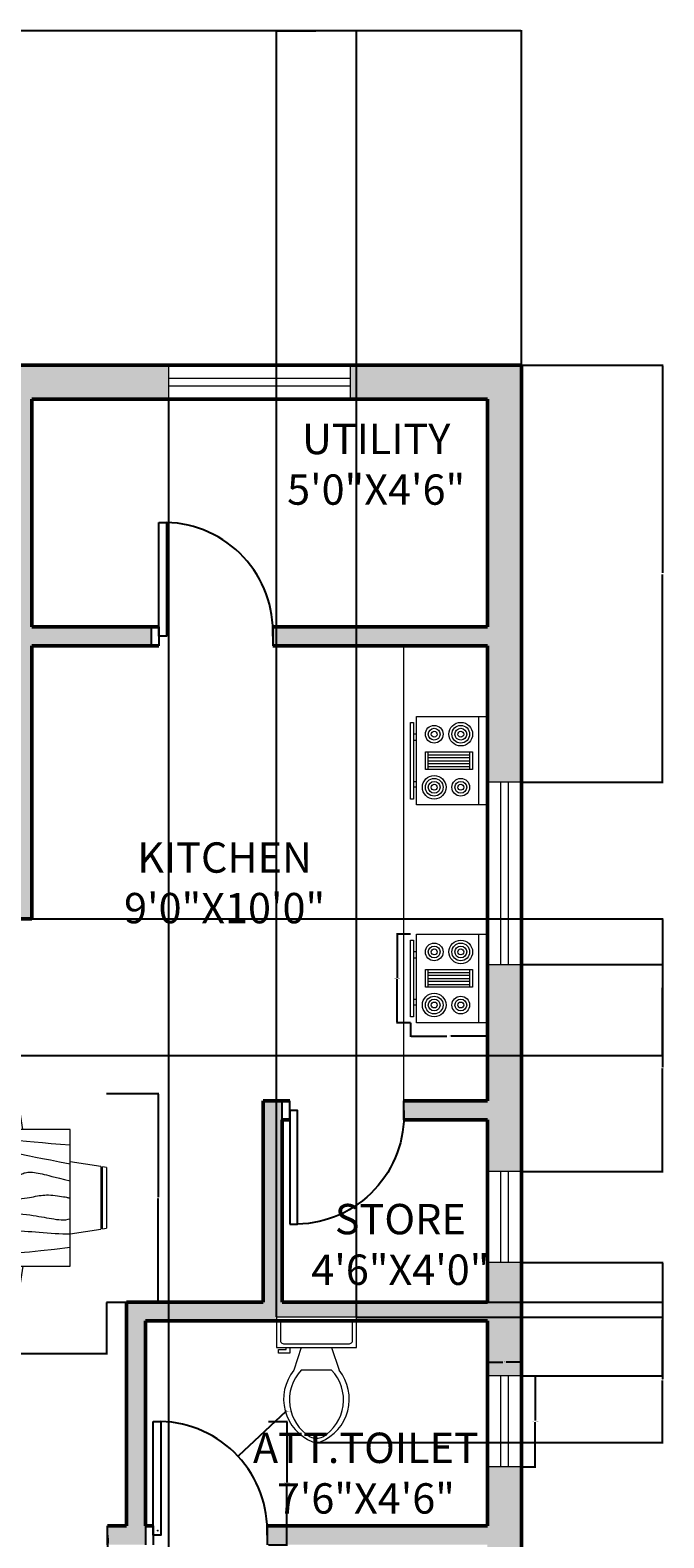
# Model space of a CAD drawing. Units: inches. Extents: x 76 to 532, y 199 to 998.
# Tile 4 of 4: x 365 to 532, y 601 to 998. Entities that reach past the tile are written whole.
import ezdxf

# ---------------------------------------------------------------- set-up
doc = ezdxf.new("R2010")
doc.units = ezdxf.units.IN
for name, color, linetype, lineweight in [('A-ANNO-DIMS', 2, 'Continuous', 18), ('A-AREA-IDEN', 3, 'Continuous', 18), ('A-EQPM', 8, 'Continuous', 18), ('A-FLOR-FIXT', 8, 'Continuous', 18), ('A-FURN', 8, 'Continuous', 18), ('A-WALL', 7, 'Continuous', 50), ('A-WALL-PATT', 45, 'Continuous', 13), ('doors', 1, 'Continuous', 25), ('windows', 140, 'Continuous', 18)]:
    doc.layers.add(name, color=color, linetype=linetype, lineweight=lineweight)
doc.styles.get("Standard").update_dxf_attribs({"font": 'arial.ttf'})
doc.dimstyles.get("Standard").update_dxf_attribs({"dimtxt": 0.18, "dimasz": 0.18, "dimexe": 0.18, "dimexo": 0.0625, "dimgap": 0.09, "dimtad": 0, "dimtih": 1, "dimtoh": 1, "dimdec": 4, "dimzin": 0, "dimdsep": 46, "dimtxsty": 'Standard', "dimcen": 0.09, "dimadec": 0, "dimazin": 0, "dimtfac": 1, "dimtdec": 4, "dimtofl": 0, "dimtmove": 0, "dimatfit": 3, "dimfxl": 1, "dimtolj": 1, "dimtzin": 0, "dimarcsym": 0})

# ---------------------------------------------------------------- blocks, each defined once
blk = doc.blocks.new('Dining Set - 36 x 72 in.')
for p, q in [((-22.2343, 26.00059), (-23.4847, 17.99762)), ((-22.2304, 26), (-5.7608, 26)), ((-22, 27.5), (-22.1562, 26.50042)), ((-5.8416, 26.5), (-22.1534, 26.5)), ((-22, 27.5), (-6, 27.5)), ((-5.8437, 26.49966), (-6, 27.5)), ((-4.5152, 17.99762), (-5.7655, 25.99926)), ((5.7657, 26.00059), (4.5153, 17.99762)), ((5.7696, 26), (22.2392, 26)), ((6, 27.5), (5.8438, 26.50042)), ((22.1584, 26.5), (5.8466, 26.5)), ((6, 27.5), (22, 27.5)), ((22.1563, 26.49966), (22, 27.5)), ((23.4848, 17.99762), (22.2345, 25.99926)), ((36, 18), (-36, 18)), ((-36, 18), (-36, -18)), ((36, -18), (36, 18)), ((-45.5, 8), (-44.5004, 8.15617)), ((-45.5, 8), (-45.5, -8)), ((-44.5, -8.15843), (-44.5, 8.15338)), ((-44.0006, 8.23428), (-35.9976, 9.48474)), ((-44, 8.23041), (-44, -8.23915)), ((44.0006, 8.23428), (35.9976, 9.48474)), ((44, 8.23041), (44, -8.23915)), ((44.5, -8.15843), (44.5, 8.15338)), ((45.5, 8), (44.5005, 8.15617)), ((45.5, 8), (45.5, -8)), ((-44.4997, -8.15631), (-45.5, -8)), ((-35.9976, -9.48476), (-43.9993, -8.2345)), ((35.9976, -9.48476), (43.9993, -8.2345)), ((44.4997, -8.15631), (45.5, -8)), ((-36, -18), (36, -18)), ((-22.2343, -26.0006), (-23.4847, -17.99762)), ((-4.5152, -17.99762), (-5.7655, -25.99928)), ((5.7657, -26.0006), (4.5153, -17.99762)), ((23.4848, -17.99762), (22.2345, -25.99928)), ((-22.2304, -26), (-5.7608, -26)), ((-22, -27.5), (-22.1562, -26.50044)), ((-5.8416, -26.5), (-22.1534, -26.5)), ((-22, -27.5), (-6, -27.5)), ((-5.8437, -26.49967), (-6, -27.5)), ((5.7696, -26), (22.2392, -26)), ((6, -27.5), (5.8438, -26.50044)), ((22.1584, -26.5), (5.8466, -26.5)), ((6, -27.5), (22, -27.5)), ((22.1563, -26.49967), (22, -27.5))]:
    blk.add_line(p, q)
for points in [[(-36, 15), (-31.1772, 14.97754), (-26.8079, 14.91406), (-22.8538, 14.81543), (-19.276, 14.6875), (-16.0362, 14.53613), (-13.0957, 14.36718), (-10.4159, 14.18652), (-7.9583, 14), (-5.6904, 13.81315), (-3.6035, 13.63021), (-1.6954, 13.45508), (0.0365, 13.29166), (1.5945, 13.14388), (2.9811, 13.01562), (4.1988, 12.9108), (5.25, 12.83333), (6.1393, 12.78613), (6.8802, 12.76823), (7.4883, 12.77767), (7.9792, 12.8125), (8.3685, 12.87077), (8.6719, 12.95052), (8.9049, 13.0498), (9.0833, 13.16666), (9.2205, 13.29899), (9.3216, 13.44401), (9.3895, 13.59879), (9.4271, 13.76041), (9.4373, 13.92594), (9.4232, 14.09245), (9.3875, 14.257), (9.3333, 14.41666), (9.2638, 14.56917), (9.1836, 14.71484), (9.0975, 14.85465), (9.0104, 14.98958), (8.9272, 15.1206), (8.8529, 15.2487), (8.7922, 15.37483), (8.75, 15.5), (8.7305, 15.62467), (8.7344, 15.74739), (8.7617, 15.86621), (8.8125, 15.97916), (8.8867, 16.08431), (8.9844, 16.17968), (9.1055, 16.26334), (9.25, 16.33333), (9.4189, 16.38802), (9.6172, 16.42708), (9.8506, 16.45052), (10.125, 16.45833), (10.4463, 16.45052), (10.8203, 16.42708), (11.2529, 16.38802), (11.75, 16.33333), (12.3184, 16.26318), (12.9694, 16.17838), (13.7151, 16.07991), (14.5677, 15.96875), (15.5395, 15.84586), (16.6426, 15.71224), (17.8893, 15.56884), (19.2917, 15.41666), (20.859, 15.25667), (22.5879, 15.08984), (24.4721, 14.91715), (26.5052, 14.73958), (28.6809, 14.5581), (30.9929, 14.3737), (33.4347, 14.18733), (36, 14)], [(-36, 10), (-28.9766, 10.14274), (-23.1725, 10.20442), (-18.4241, 10.19775), (-14.5677, 10.13541), (-11.4399, 10.03011), (-8.877, 9.89453), (-6.7154, 9.74137), (-4.7917, 9.58333), (-2.9698, 9.43082), (-1.2246, 9.28515), (0.4415, 9.14534), (2.026, 9.01041), (3.5266, 8.87939), (4.9408, 8.7513), (6.266, 8.62516), (7.5, 8.5), (8.6411, 8.37549), (9.6914, 8.2539), (10.6538, 8.13818), (11.5312, 8.03125), (12.3267, 7.93603), (13.043, 7.85547), (13.6831, 7.79248), (14.25, 7.75), (14.7471, 7.7303), (15.1797, 7.73307), (15.5537, 7.75732), (15.875, 7.80208), (16.1494, 7.86637), (16.3828, 7.94922), (16.5811, 8.04964), (16.75, 8.16666), (16.8944, 8.29915), (17.0143, 8.44531), (17.1089, 8.60319), (17.1771, 8.77083), (17.218, 8.94629), (17.2305, 9.1276), (17.2137, 9.31282), (17.1667, 9.5), (17.0895, 9.6875), (16.987, 9.875), (16.8649, 10.0625), (16.7292, 10.25), (16.5856, 10.4375), (16.4401, 10.625), (16.2985, 10.8125), (16.1667, 11), (16.05, 11.18733), (15.9518, 11.3737), (15.8752, 11.5581), (15.8229, 11.73958), (15.798, 11.91715), (15.8034, 12.08984), (15.842, 12.25667), (15.9167, 12.41666), (16.0295, 12.56836), (16.1784, 12.70833), (16.3605, 12.83268), (16.5729, 12.9375), (16.8127, 13.01888), (17.0768, 13.07291), (17.3625, 13.0957), (17.6667, 13.08333), (17.9894, 13.03312), (18.3418, 12.94726), (18.7382, 12.82918), (19.1927, 12.68229), (19.7195, 12.51001), (20.3327, 12.31575), (21.0465, 12.10294), (21.875, 11.875), (22.8357, 11.63354), (23.959, 11.37304), (25.2786, 11.08618), (26.8282, 10.76562), (28.6414, 10.40405), (30.752, 9.99414), (33.1936, 9.52856), (36, 9)], [(-36, 5.5), (-30.7157, 5.3348), (-26.069, 5.20963), (-21.9946, 5.11767), (-18.4271, 5.05208), (-15.3009, 5.00602), (-12.5508, 4.97265), (-10.1112, 4.94515), (-7.9167, 4.91666), (-5.909, 4.88167), (-4.0586, 4.83984), (-2.3429, 4.79215), (-0.7396, 4.73958), (0.7739, 4.6831), (2.22, 4.6237), (3.6213, 4.56233), (5, 4.5), (6.373, 4.43782), (7.7344, 4.3776), (9.0723, 4.32129), (10.375, 4.27083), (11.6309, 4.22819), (12.8281, 4.19531), (13.9551, 4.17415), (15, 4.16666), (15.954, 4.17448), (16.819, 4.19791), (17.6001, 4.23698), (18.3021, 4.29166), (18.9299, 4.36198), (19.4883, 4.44791), (19.9823, 4.54948), (20.4167, 4.66666), (20.7969, 4.79899), (21.1302, 4.94401), (21.4245, 5.09879), (21.6875, 5.26041), (21.9271, 5.42594), (22.1511, 5.59245), (22.3672, 5.757), (22.5834, 5.91666), (22.8065, 6.06868), (23.0404, 6.21093), (23.2879, 6.34147), (23.5521, 6.45833), (23.8358, 6.55957), (24.142, 6.64323), (24.4735, 6.70735), (24.8334, 6.75), (25.2235, 6.76969), (25.642, 6.76692), (26.0858, 6.74267), (26.5521, 6.69791), (27.0379, 6.63362), (27.5404, 6.55078), (28.0565, 6.45036), (28.5834, 6.33333), (29.1242, 6.19987), (29.7071, 6.04687), (30.3661, 5.87044), (31.1354, 5.66666), (32.0493, 5.43164), (33.142, 5.16146), (34.4475, 4.85221), (36, 4.5)], [(-36, -1), (-30.7915, -0.6591), (-26.0195, -0.38216), (-21.6519, -0.16284), (-17.6563, 0.00521), (-14.0005, 0.12833), (-10.6523, 0.21289), (-7.5796, 0.26522), (-4.75, 0.29166), (-2.134, 0.29793), (0.2878, 0.28711), (2.5317, 0.26163), (4.6146, 0.22396), (6.5529, 0.17651), (8.3633, 0.12174), (10.0623, 0.06209), (11.6667, 0), (13.1899, -0.06201), (14.6341, -0.1211), (15.9982, -0.17432), (17.2813, -0.21875), (18.4823, -0.25147), (19.6003, -0.26953), (20.6343, -0.27002), (21.5834, -0.25), (22.4481, -0.20768), (23.2357, -0.14584), (23.9549, -0.06836), (24.6146, 0.02083), (25.2235, 0.11784), (25.7904, 0.21875), (26.3241, 0.31966), (26.8334, 0.41666), (27.3265, 0.50618), (27.8099, 0.58593), (28.2894, 0.65397), (28.7709, 0.70833), (29.2601, 0.74707), (29.763, 0.76823), (30.2855, 0.76985), (30.8334, 0.75), (31.4088, 0.70784), (31.9994, 0.64713), (32.589, 0.57275), (33.1615, 0.48958), (33.7008, 0.4025), (34.1908, 0.3164), (34.6153, 0.23616), (34.9584, 0.16666), (35.2099, 0.11165), (35.3848, 0.07031), (35.504, 0.04069), (35.5886, 0.02083), (35.6594, 0.00879), (35.7377, 0.0026), (35.8442, 0.00032), (36, 0)], [(-36, -6.5), (-27.1843, -6.31267), (-20.084, -6.1263), (-14.469, -5.9419), (-10.1094, -5.76042), (-6.7752, -5.58285), (-4.2363, -5.41016), (-2.2629, -5.24333), (-0.625, -5.08334), (0.8708, -4.93099), (2.2715, -4.78646), (3.5872, -4.64974), (4.8281, -4.52084), (6.0046, -4.39974), (7.127, -4.28646), (8.2053, -4.18099), (9.25, -4.08334), (10.2705, -3.99382), (11.2734, -3.91407), (12.2647, -3.84603), (13.25, -3.79167), (14.2354, -3.75293), (15.2266, -3.73177), (16.2295, -3.73015), (17.25, -3.75), (18.2912, -3.79248), (19.3451, -3.85547), (20.4009, -3.93604), (21.4479, -4.03125), (22.4754, -4.13819), (23.4727, -4.25391), (24.4289, -4.37549), (25.3334, -4.5), (26.1785, -4.62492), (26.9694, -4.74935), (27.7145, -4.87281), (28.4219, -4.99479), (29.1, -5.11483), (29.7572, -5.23242), (30.4016, -5.34709), (31.0417, -5.45834), (31.6837, -5.56437), (32.3262, -5.65821), (32.9658, -5.73153), (33.599, -5.77604), (34.2224, -5.78345), (34.8327, -5.74545), (35.4264, -5.65373), (36, -5.5)], [(-36, -10), (-26.4022, -9.81299), (-18.4675, -9.62891), (-11.9839, -9.45069), (-6.7396, -9.28125), (-2.5226, -9.12354), (0.8789, -8.98047), (3.6769, -8.85498), (6.0833, -8.75), (8.2767, -8.66765), (10.3021, -8.60677), (12.1712, -8.56543), (13.8958, -8.54167), (15.4876, -8.53353), (16.9583, -8.53907), (18.3197, -8.55632), (19.5834, -8.58334), (20.7616, -8.61841), (21.8685, -8.66081), (22.9188, -8.71004), (23.9271, -8.76563), (24.9081, -8.82707), (25.8763, -8.89388), (26.8465, -8.96558), (27.8334, -9.04167), (28.8474, -9.12118), (29.8828, -9.20117), (30.93, -9.27824), (31.9792, -9.34896), (33.0205, -9.40991), (34.0443, -9.45768), (35.0407, -9.48885), (36, -9.5)], [(-36, -14.5), (-30.0881, -14.33513), (-25.0332, -14.21224), (-20.7312, -14.12647), (-17.0781, -14.07292), (-13.97, -14.04671), (-11.3027, -14.04297), (-8.9724, -14.05681), (-6.875, -14.08334), (-4.9224, -14.11833), (-3.0905, -14.16016), (-1.3709, -14.20785), (0.2448, -14.26042), (1.7647, -14.3169), (3.1973, -14.3763), (4.5507, -14.43767), (5.8333, -14.5), (7.0554, -14.5621), (8.235, -14.62175), (9.3922, -14.67652), (10.5469, -14.72396), (11.7192, -14.76164), (12.929, -14.78711), (14.1965, -14.79794), (15.5417, -14.79167), (16.9933, -14.76424), (18.6152, -14.70508), (20.4804, -14.60197), (22.6615, -14.44271), (25.2312, -14.21509), (28.2624, -13.9069), (31.8277, -13.50594), (36, -13)]]:
    blk.add_lwpolyline(points)
blk = doc.blocks.new('Range-Oven - 30 in top')
for p, q in [((0, -3), (30, -3)), ((12, -6), (18, -6)), ((13, -20), (13, -6)), ((14, -6), (14, -20)), ((15, -20), (15, -6)), ((16, -6), (16, -20)), ((17, -20), (17, -6)), ((18, -20), (12, -20)), ((6, -24), (6, -25)), ((8, -25), (8, -24)), ((22, -25), (22, -24)), ((24, -24), (24, -25))]:
    blk.add_line(p, q)
for points in [[(0, -24), (0, 0), (30, 0), (30, -24)], [(12, -21), (12, -5), (18, -5), (18, -21)], [(2, -26), (2, -25), (28, -25), (28, -26)]]:
    blk.add_lwpolyline(points, close=True)
for centre, radius in [((6, -9), 4), ((6, -9), 3), ((6, -9), 2), ((6, -9), 1), ((24, -9), 3), ((24, -9), 2), ((24, -9), 1), ((6, -18), 3), ((24, -18), 4), ((24, -18), 3), ((6, -18), 2), ((6, -18), 1), ((24, -18), 2), ((24, -18), 1)]:
    blk.add_circle(centre, radius)
blk = doc.blocks.new('*U10')
for p, q in [((9.5, -6), (9.5, -2)), ((-10, -8.5), (-8, -8.5)), ((-10, -9.5), (-10, -8.5)), ((-7, -9.5), (-10, -9.5)), ((-8, -8.5), (-8, -8)), ((-7, -8), (-7, -9.5)), ((-4, -8), (-6, -14)), ((4, -8), (6, -14)), ((4, -14), (-4, -14))]:
    blk.add_line(p, q)
blk.add_lwpolyline([(10.5, -8), (10.5, 0), (-10.5, 0), (-10.5, -8)], close=True)
for points in [[(-9.5, -2), (-9.5, -6)], [(8.5, -1), (-8.5, -1)], [(-8.5, -7), (8.5, -7)]]:
    blk.add_lwpolyline(points)
for centre, radius, start, end in [((-8.62, -1.88), 0.884, 81.8699, 188.1301), ((8.62, -1.88), 0.884, 351.8699, 98.1301), ((-8.62, -6.12), 0.884, 171.8699, 278.1301), ((8.62, -6.12), 0.884, 261.8699, 8.1301), ((3.52, -21.58), 12.17, 141.4691, 247.9714), ((4.2, -21.82), 11.33, 136.3677, 238.9468), ((-3.52, -21.58), 12.17, 292.0284, 38.5307), ((-4.2, -21.82), 11.33, 301.053, 43.6321), ((0, -27.88), 4, 245.7318, 294.2682), ((0, -29), 4, 254.8605, 285.1395)]:
    blk.add_arc(centre, radius, start, end)
blk = doc.blocks.new('glass')
at = {"layer": 'windows'}
for p, q in [((-12, 5.5), (-12, -3.5)), ((12, 5.5), (12, -3.5)), ((-12, 2), (12, 2)), ((-12, 0), (12, 0))]:
    blk.add_line(p, q, dxfattribs=at)
blk = doc.blocks.new('DOOR-SWING-30IN')
for p, q in [((0, 5), (0, 0)), ((2, 5), (2, 0)), ((32, 5), (32, 0))]:
    blk.add_line(p, q)
blk.add_lwpolyline([(2, 32.5), (4, 32.5), (4, 2.5), (2, 2.5)], close=True)
blk.add_arc((3.27, 3.75), 28.76, 357.5089, 88.5412)
blk = doc.blocks.new('WIN-48IN')
for p, q in [((0, 5.5), (48, 5.5)), ((0, 3.5), (48, 3.5))]:
    blk.add_line(p, q)
blk.add_lwpolyline([(0, 0), (48, 0), (48, 9), (0, 9)], close=True)
blk = doc.blocks.new('*D15')
at = {"layer": 'A-ANNO-DIMS', "color": 0, "lineweight": -2, "transparency": 16777216}
for p, q in [((428.25, 631.53), (433.25, 631.53)), ((433.07, 631.35), (433.07, 615.46)), ((433.07, 599.21), (433.07, 615.09)), ((428.25, 599.03), (433.25, 599.03))]:
    blk.add_line(p, q, dxfattribs=at)
at = {"layer": 'A-ANNO-DIMS', "color": 0, "transparency": 16777216}
for points in [[(433.04, 631.35), (433.1, 631.35), (433.07, 631.53)], [(433.04, 599.21), (433.1, 599.21), (433.07, 599.03)]]:
    blk.add_solid(points, dxfattribs=at)
at = {"layer": 'Defpoints', "color": 0, "transparency": 16777216}
for p in [(428.19, 631.53), (433.07, 631.53), (428.19, 599.03)]:
    blk.add_point(p, dxfattribs=at)
at = {"layer": 'A-ANNO-DIMS', "color": 0, "transparency": 16777216, "insert": (433.07, 615.28), "char_height": 0.18, "attachment_point": 5}
blk.add_mtext('\\A1;DOOR 33 TYP.', dxfattribs=at)
blk = doc.blocks.new('*D19')
at = {"layer": 'A-ANNO-DIMS', "color": 0, "lineweight": -2, "transparency": 16777216}
for p, q in [((494.92, 643.58), (498.64, 643.58)), ((498.46, 643.4), (498.46, 631.76)), ((498.46, 619.76), (498.46, 631.39)), ((494.92, 619.58), (498.64, 619.58))]:
    blk.add_line(p, q, dxfattribs=at)
at = {"layer": 'A-ANNO-DIMS', "color": 0, "transparency": 16777216}
for points in [[(498.43, 643.4), (498.49, 643.4), (498.46, 643.58)], [(498.43, 619.76), (498.49, 619.76), (498.46, 619.58)]]:
    blk.add_solid(points, dxfattribs=at)
at = {"layer": 'Defpoints', "color": 0, "transparency": 16777216}
for p in [(494.86, 643.58), (494.86, 619.58), (498.46, 619.58)]:
    blk.add_point(p, dxfattribs=at)
at = {"layer": 'A-ANNO-DIMS', "color": 0, "transparency": 16777216, "insert": (498.46, 631.58), "char_height": 0.18, "attachment_point": 5}
blk.add_mtext('\\A1;GLAZING 24 TYP.', dxfattribs=at)
blk = doc.blocks.new('*D20')
at = {"layer": 'A-ANNO-DIMS', "color": 0, "lineweight": -2, "transparency": 16777216}
for p, q in [((485.86, 643.64), (485.86, 647.36)), ((486.04, 647.18), (489.9, 647.18)), ((494.68, 647.18), (490.82, 647.18)), ((494.86, 643.64), (494.86, 647.36))]:
    blk.add_line(p, q, dxfattribs=at)
at = {"layer": 'A-ANNO-DIMS', "color": 0, "transparency": 16777216}
for points in [[(486.04, 647.21), (486.04, 647.15), (485.86, 647.18)], [(494.68, 647.21), (494.68, 647.15), (494.86, 647.18)]]:
    blk.add_solid(points, dxfattribs=at)
at = {"layer": 'Defpoints', "color": 0, "transparency": 16777216}
for p in [(494.86, 647.18), (485.86, 643.58), (494.86, 643.58)]:
    blk.add_point(p, dxfattribs=at)
at = {"layer": 'A-ANNO-DIMS', "color": 0, "transparency": 16777216, "insert": (490.36, 647.18), "char_height": 0.18, "attachment_point": 5}
blk.add_mtext('\\A1;9 TYP.', dxfattribs=at)
blk = doc.blocks.new('*D23')
at = {"layer": 'A-ANNO-DIMS', "color": 0, "lineweight": -2, "transparency": 16777216}
for p, q in [((465.58, 759.98), (461.96, 759.98)), ((462.14, 759.8), (462.14, 748.5)), ((462.14, 736.83), (462.14, 748.13)), ((465.58, 736.65), (461.96, 736.65))]:
    blk.add_line(p, q, dxfattribs=at)
at = {"layer": 'A-ANNO-DIMS', "color": 0, "transparency": 16777216}
for points in [[(462.11, 759.8), (462.17, 759.8), (462.14, 759.98)], [(462.11, 736.83), (462.17, 736.83), (462.14, 736.65)]]:
    blk.add_solid(points, dxfattribs=at)
at = {"layer": 'Defpoints', "color": 0, "transparency": 16777216}
for p in [(465.64, 759.98), (462.14, 736.65), (465.64, 736.65)]:
    blk.add_point(p, dxfattribs=at)
at = {"layer": 'A-ANNO-DIMS', "color": 0, "transparency": 16777216, "insert": (462.14, 748.31), "char_height": 0.18, "attachment_point": 5}
blk.add_mtext('\\A1;RANGE 23 TYP.', dxfattribs=at)
blk = doc.blocks.new('*D24')
at = {"layer": 'A-ANNO-DIMS', "color": 0, "lineweight": -2, "transparency": 16777216}
for p, q in [((465.64, 736.59), (465.64, 732.97)), ((485.86, 736.59), (485.86, 732.97)), ((465.82, 733.15), (475.22, 733.15)), ((485.68, 733.15), (476.28, 733.15))]:
    blk.add_line(p, q, dxfattribs=at)
at = {"layer": 'A-ANNO-DIMS', "color": 0, "transparency": 16777216}
for points in [[(465.82, 733.18), (465.82, 733.12), (465.64, 733.15)], [(485.68, 733.18), (485.68, 733.12), (485.86, 733.15)]]:
    blk.add_solid(points, dxfattribs=at)
at = {"layer": 'Defpoints', "color": 0, "transparency": 16777216}
for p in [(465.64, 736.65), (485.86, 736.65), (485.86, 733.15)]:
    blk.add_point(p, dxfattribs=at)
at = {"layer": 'A-ANNO-DIMS', "color": 0, "transparency": 16777216, "insert": (475.75, 733.15), "char_height": 0.18, "attachment_point": 5}
blk.add_mtext('\\A1;20 TYP.', dxfattribs=at)
blk = doc.blocks.new('*D29')
at = {"layer": 'A-ANNO-DIMS', "color": 0, "lineweight": -2, "transparency": 16777216}
for p, q in [((294.53, 662.92), (294.53, 649.15)), ((385.53, 662.92), (385.53, 649.15)), ((294.71, 649.33), (339.08, 649.33)), ((385.35, 649.33), (340.98, 649.33))]:
    blk.add_line(p, q, dxfattribs=at)
at = {"layer": 'A-ANNO-DIMS', "color": 0, "transparency": 16777216}
for points in [[(294.71, 649.36), (294.71, 649.3), (294.53, 649.33)], [(385.35, 649.36), (385.35, 649.3), (385.53, 649.33)]]:
    blk.add_solid(points, dxfattribs=at)
at = {"layer": 'Defpoints', "color": 0, "transparency": 16777216}
for p in [(294.53, 662.98), (385.53, 662.98), (385.53, 649.33)]:
    blk.add_point(p, dxfattribs=at)
at = {"layer": 'A-ANNO-DIMS', "color": 0, "transparency": 16777216, "insert": (340.03, 649.33), "char_height": 0.18, "attachment_point": 5}
blk.add_mtext('\\A1;DINING SET 91', dxfattribs=at)
blk = doc.blocks.new('*D30')
at = {"layer": 'A-ANNO-DIMS', "color": 0, "lineweight": -2, "transparency": 16777216}
for p, q in [((385.59, 717.98), (399.36, 717.98)), ((399.18, 717.8), (399.18, 690.66)), ((399.18, 663.16), (399.18, 690.3)), ((385.59, 662.98), (399.36, 662.98))]:
    blk.add_line(p, q, dxfattribs=at)
at = {"layer": 'A-ANNO-DIMS', "color": 0, "transparency": 16777216}
for points in [[(399.15, 717.8), (399.21, 717.8), (399.18, 717.98)], [(399.15, 663.16), (399.21, 663.16), (399.18, 662.98)]]:
    blk.add_solid(points, dxfattribs=at)
at = {"layer": 'Defpoints', "color": 0, "transparency": 16777216}
for p in [(385.53, 717.98), (399.18, 717.98), (385.53, 662.98)]:
    blk.add_point(p, dxfattribs=at)
at = {"layer": 'A-ANNO-DIMS', "color": 0, "transparency": 16777216, "insert": (399.18, 690.48), "char_height": 0.18, "attachment_point": 5}
blk.add_mtext('\\A1;55', dxfattribs=at)
blk = doc.blocks.new('*D31')
at = {"layer": 'A-ANNO-DIMS', "color": 0, "lineweight": -2, "transparency": 16777216}
for p, q in [((160.86, 910.09), (160.86, 998.31)), ((161.04, 998.13), (327.57, 998.13)), ((494.68, 998.13), (328.15, 998.13)), ((494.86, 910.09), (494.86, 998.31))]:
    blk.add_line(p, q, dxfattribs=at)
at = {"layer": 'A-ANNO-DIMS', "color": 0, "transparency": 16777216}
for points in [[(161.04, 998.16), (161.04, 998.1), (160.86, 998.13)], [(494.68, 998.16), (494.68, 998.1), (494.86, 998.13)]]:
    blk.add_solid(points, dxfattribs=at)
at = {"layer": 'Defpoints', "color": 0, "transparency": 16777216}
for p in [(494.86, 998.13), (160.86, 910.03), (494.86, 910.03)]:
    blk.add_point(p, dxfattribs=at)
at = {"layer": 'A-ANNO-DIMS', "color": 0, "transparency": 16777216, "insert": (327.86, 998.13), "char_height": 0.18, "attachment_point": 5}
blk.add_mtext('\\A1;334', dxfattribs=at)
blk = doc.blocks.new('*D34')
at = {"layer": 'A-ANNO-DIMS', "color": 0, "lineweight": -2, "transparency": 16777216}
for p, q in [((494.92, 910.03), (532.14, 910.03)), ((531.96, 909.85), (531.96, 855.21)), ((531.96, 800.21), (531.96, 854.85)), ((494.92, 800.03), (532.14, 800.03))]:
    blk.add_line(p, q, dxfattribs=at)
at = {"layer": 'A-ANNO-DIMS', "color": 0, "transparency": 16777216}
for points in [[(531.93, 909.85), (531.99, 909.85), (531.96, 910.03)], [(531.93, 800.21), (531.99, 800.21), (531.96, 800.03)]]:
    blk.add_solid(points, dxfattribs=at)
at = {"layer": 'Defpoints', "color": 0, "transparency": 16777216}
for p in [(494.86, 910.03), (531.96, 910.03), (494.86, 800.03)]:
    blk.add_point(p, dxfattribs=at)
at = {"layer": 'A-ANNO-DIMS', "color": 0, "transparency": 16777216, "insert": (531.96, 855.03), "char_height": 0.18, "attachment_point": 5}
blk.add_mtext('\\A1;110', dxfattribs=at)
blk = doc.blocks.new('*D35')
at = {"layer": 'A-ANNO-DIMS', "color": 0, "lineweight": -2, "transparency": 16777216}
for p, q in [((494.92, 752.03), (532.14, 752.03)), ((531.96, 751.85), (531.96, 724.93)), ((531.96, 697.65), (531.96, 724.57)), ((494.92, 697.47), (532.14, 697.47))]:
    blk.add_line(p, q, dxfattribs=at)
at = {"layer": 'A-ANNO-DIMS', "color": 0, "transparency": 16777216}
for points in [[(531.93, 751.85), (531.99, 751.85), (531.96, 752.03)], [(531.93, 697.65), (531.99, 697.65), (531.96, 697.47)]]:
    blk.add_solid(points, dxfattribs=at)
at = {"layer": 'Defpoints', "color": 0, "transparency": 16777216}
for p in [(494.86, 752.03), (531.96, 752.03), (494.86, 697.47)]:
    blk.add_point(p, dxfattribs=at)
at = {"layer": 'A-ANNO-DIMS', "color": 0, "transparency": 16777216, "insert": (531.96, 724.75), "char_height": 0.18, "attachment_point": 5}
blk.add_mtext('\\A1;54.55', dxfattribs=at)
blk = doc.blocks.new('*D36')
at = {"layer": 'A-ANNO-DIMS', "color": 0, "lineweight": -2, "transparency": 16777216}
for p, q in [((494.92, 673.47), (532.14, 673.47)), ((531.96, 673.29), (531.96, 658.71)), ((531.96, 643.76), (531.96, 658.34)), ((494.92, 643.58), (532.14, 643.58))]:
    blk.add_line(p, q, dxfattribs=at)
at = {"layer": 'A-ANNO-DIMS', "color": 0, "transparency": 16777216}
for points in [[(531.93, 673.29), (531.99, 673.29), (531.96, 673.47)], [(531.93, 643.76), (531.99, 643.76), (531.96, 643.58)]]:
    blk.add_solid(points, dxfattribs=at)
at = {"layer": 'Defpoints', "color": 0, "transparency": 16777216}
for p in [(494.86, 673.47), (494.86, 643.58), (531.96, 643.58)]:
    blk.add_point(p, dxfattribs=at)
at = {"layer": 'A-ANNO-DIMS', "color": 0, "transparency": 16777216, "insert": (531.96, 658.53), "char_height": 0.18, "attachment_point": 5}
blk.add_mtext('\\A1;29.895', dxfattribs=at)
blk = doc.blocks.new('*D41')
at = {"layer": 'A-ANNO-DIMS', "color": 0, "lineweight": -2, "transparency": 16777216}
for p, q in [((347.36, 900.97), (347.36, 198.6)), ((401.86, 900.97), (401.86, 198.6)), ((347.54, 198.78), (374.28, 198.78)), ((401.68, 198.78), (374.93, 198.78))]:
    blk.add_line(p, q, dxfattribs=at)
at = {"layer": 'A-ANNO-DIMS', "color": 0, "transparency": 16777216}
for points in [[(347.54, 198.81), (347.54, 198.75), (347.36, 198.78)], [(401.68, 198.81), (401.68, 198.75), (401.86, 198.78)]]:
    blk.add_solid(points, dxfattribs=at)
at = {"layer": 'Defpoints', "color": 0, "transparency": 16777216}
for p in [(347.36, 901.03), (401.86, 901.03), (401.86, 198.78)]:
    blk.add_point(p, dxfattribs=at)
at = {"layer": 'A-ANNO-DIMS', "color": 0, "transparency": 16777216, "insert": (374.61, 198.78), "char_height": 0.18, "attachment_point": 5}
blk.add_mtext('\\A1;54.5', dxfattribs=at)
blk = doc.blocks.new('*D46')
at = {"layer": 'A-ANNO-DIMS', "color": 0, "lineweight": -2, "transparency": 16777216}
for p, q in [((249.92, 764.03), (532.14, 764.03)), ((531.96, 763.85), (531.96, 746.21)), ((531.96, 728.21), (531.96, 745.85)), ((249.92, 728.03), (532.14, 728.03))]:
    blk.add_line(p, q, dxfattribs=at)
at = {"layer": 'A-ANNO-DIMS', "color": 0, "transparency": 16777216}
for points in [[(531.93, 763.85), (531.99, 763.85), (531.96, 764.03)], [(531.93, 728.21), (531.99, 728.21), (531.96, 728.03)]]:
    blk.add_solid(points, dxfattribs=at)
at = {"layer": 'Defpoints', "color": 0, "transparency": 16777216}
for p in [(249.86, 764.03), (531.96, 764.03), (249.86, 728.03)]:
    blk.add_point(p, dxfattribs=at)
at = {"layer": 'A-ANNO-DIMS', "color": 0, "transparency": 16777216, "insert": (531.96, 746.03), "char_height": 0.18, "attachment_point": 5}
blk.add_mtext('\\A1;36', dxfattribs=at)
blk = doc.blocks.new('*D48')
at = {"layer": 'A-ANNO-DIMS', "color": 0, "lineweight": -2, "transparency": 16777216}
for p, q in [((430.36, 659.09), (430.36, 998.31)), ((430.54, 998.13), (440.65, 998.13)), ((451.18, 998.13), (441.06, 998.13)), ((451.36, 659.09), (451.36, 998.31))]:
    blk.add_line(p, q, dxfattribs=at)
at = {"layer": 'A-ANNO-DIMS', "color": 0, "transparency": 16777216}
for points in [[(430.54, 998.16), (430.54, 998.1), (430.36, 998.13)], [(451.18, 998.16), (451.18, 998.1), (451.36, 998.13)]]:
    blk.add_solid(points, dxfattribs=at)
at = {"layer": 'Defpoints', "color": 0, "transparency": 16777216}
for p in [(451.36, 998.13), (430.36, 659.03), (451.36, 659.03)]:
    blk.add_point(p, dxfattribs=at)
at = {"layer": 'A-ANNO-DIMS', "color": 0, "transparency": 16777216, "insert": (440.86, 998.13), "char_height": 0.18, "attachment_point": 5}
blk.add_mtext('\\A1;21', dxfattribs=at)
blk = doc.blocks.new('*D49')
at = {"layer": 'A-ANNO-DIMS', "color": 0, "lineweight": -2, "transparency": 16777216}
for p, q in [((485.92, 663.03), (532.14, 663.03)), ((531.96, 662.85), (531.96, 653.48)), ((531.96, 643.76), (531.96, 653.12)), ((494.92, 643.58), (532.14, 643.58))]:
    blk.add_line(p, q, dxfattribs=at)
at = {"layer": 'A-ANNO-DIMS', "color": 0, "transparency": 16777216}
for points in [[(531.93, 662.85), (531.99, 662.85), (531.96, 663.03)], [(531.93, 643.76), (531.99, 643.76), (531.96, 643.58)]]:
    blk.add_solid(points, dxfattribs=at)
at = {"layer": 'Defpoints', "color": 0, "transparency": 16777216}
for p in [(485.86, 663.03), (531.96, 663.03), (494.86, 643.58)]:
    blk.add_point(p, dxfattribs=at)
at = {"layer": 'A-ANNO-DIMS', "color": 0, "transparency": 16777216, "insert": (531.96, 653.3), "char_height": 0.18, "attachment_point": 5}
blk.add_mtext('\\A1;19.45', dxfattribs=at)
blk = doc.blocks.new('*D55')
at = {"layer": 'A-ANNO-DIMS', "color": 0, "lineweight": -2, "transparency": 16777216}
for p, q in [((451.42, 659.03), (532.14, 659.03)), ((531.96, 658.85), (531.96, 642.71)), ((531.96, 626.21), (531.96, 642.35)), ((440.92, 626.03), (532.14, 626.03))]:
    blk.add_line(p, q, dxfattribs=at)
at = {"layer": 'A-ANNO-DIMS', "color": 0, "transparency": 16777216}
for points in [[(531.93, 658.85), (531.99, 658.85), (531.96, 659.03)], [(531.93, 626.21), (531.99, 626.21), (531.96, 626.03)]]:
    blk.add_solid(points, dxfattribs=at)
at = {"layer": 'Defpoints', "color": 0, "transparency": 16777216}
for p in [(451.36, 659.03), (440.86, 626.03), (531.96, 626.03)]:
    blk.add_point(p, dxfattribs=at)
at = {"layer": 'A-ANNO-DIMS', "color": 0, "transparency": 16777216, "insert": (531.96, 642.53), "char_height": 0.18, "attachment_point": 5}
blk.add_mtext('\\A1;33', dxfattribs=at)
blk = doc.blocks.new('*D60')
at = {"layer": 'A-ANNO-DIMS', "color": 0, "lineweight": -2, "transparency": 16777216}
for p, q in [((432.76, 634.17), (420.28, 622.52)), ((432.94, 634.17), (432.76, 634.17)), ((399.03, 602.78), (399.21, 602.78)), ((399.12, 602.69), (399.12, 602.87))]:
    blk.add_line(p, q, dxfattribs=at)
at = {"layer": 'A-ANNO-DIMS', "color": 0, "transparency": 16777216}
blk.add_solid([(420.26, 622.55), (420.3, 622.5), (420.15, 622.4)], dxfattribs=at)
at = {"layer": 'Defpoints', "color": 0, "transparency": 16777216}
for p in [(420.15, 622.4), (399.12, 602.78)]:
    blk.add_point(p, dxfattribs=at)
at = {"layer": 'A-ANNO-DIMS', "color": 0, "transparency": 16777216, "insert": (433.62, 634.17), "char_height": 0.18, "attachment_point": 5}
blk.add_mtext('\\A1;3X R28.76', dxfattribs=at)

msp = doc.modelspace()

# ---------------------------------------------------------------- hatches: boundary and pattern name
at = {"layer": 'A-WALL-PATT'}
h = msp.add_hatch(color=256, dxfattribs=at)
h.dxf.hatch_style = 1
h.paths.add_polyline_path([(323.3571, 910.0275), (259.8571, 910.0275), (259.8571, 901.0275), (301.8571, 901.0275), (301.8571, 769.0275), (301.8571, 764.0275), (306.8571, 764.0275), (306.8571, 806.0275), (306.8571, 811.0275), (306.8571, 901.0275), (323.3571, 901.0275)])
h.paths.add_polyline_path([(211.8571, 910.0275), (160.8571, 910.0275), (160.8571, 539.5719), (169.8571, 539.5719), (169.8571, 599.0275), (263.8571, 599.0275), (263.8571, 604.0275), (169.8571, 604.0275), (169.8571, 764.0275), (263.8571, 764.0275), (263.8571, 766.5275, -0.0179874), (263.8571, 769.0275), (169.8571, 769.0275), (169.8571, 901.0275), (211.8571, 901.0275)])
h.paths.add_polyline_path([(401.8571, 910.0275), (347.3571, 910.0275), (347.3571, 901.0275), (360.8571, 901.0275), (360.8571, 811.0275), (338.8571, 811.0275, -0.02174236), (338.8571, 808.5275), (338.8571, 806.0275), (360.8571, 806.0275), (360.8571, 764.0275), (365.8571, 764.0275), (365.8571, 836.0275), (397.3621, 836.0275), (397.3621, 841.0275), (365.8571, 841.0275), (365.8571, 901.0275), (401.8571, 901.0275)])
h.paths.add_polyline_path([(169.8571, 479.5719), (160.8571, 479.5719), (160.8571, 434.0275), (211.8571, 434.0275), (211.8571, 443.0275), (169.8571, 443.0275)])
h.paths.add_polyline_path([(310.8571, 443.0275), (259.8571, 443.0275), (259.8571, 434.0275), (310.8571, 434.0275), (310.8571, 438.5275, -0.03336892)])
h.paths.add_polyline_path([(353.8571, 599.0275), (353.8571, 604.0275), (348.8571, 604.0275), (348.8571, 599.0275), (348.8571, 443.0275), (348.8571, 434.0275), (396.8571, 434.0275), (396.8571, 443.0275), (353.8571, 443.0275)])
h.paths.add_polyline_path([(494.8571, 619.5776), (485.8571, 619.5776), (485.8571, 604.0275), (427.8571, 604.0275, -0.02174236), (427.8571, 601.5275), (427.8571, 599.0275), (485.8571, 599.0275), (485.8571, 443.0275), (444.8571, 443.0275), (444.8571, 434.0275), (494.8571, 434.0275)])
h.paths.add_polyline_path([(494.8571, 673.4729), (485.8571, 673.4729), (485.8571, 663.0275), (431.8571, 663.0275), (431.8571, 711.0275), (431.8571, 716.0275), (426.8571, 716.0275), (426.8571, 663.0275), (390.8571, 663.0275), (390.8571, 604.0275), (385.8571, 604.0275), (385.8571, 601.5275, -0.02174236), (385.8571, 599.0275), (395.8571, 599.0275), (395.8571, 604.0275), (395.8571, 658.0275), (430.3571, 658.0275), (430.3571, 659.0275), (451.3571, 659.0275), (451.3571, 658.0275), (485.8571, 658.0275), (485.8571, 643.5776), (494.8571, 643.5776)])
h.paths.add_polyline_path([(494.8571, 752.0275), (485.8571, 752.0275), (485.8571, 716.0275), (463.8571, 716.0275), (463.8571, 713.5275, -0.02174236), (463.8571, 711.0275), (485.8571, 711.0275), (485.8571, 697.4729), (494.8571, 697.4729)])
h.paths.add_polyline_path([(494.8571, 910.0275), (449.8571, 910.0275), (449.8571, 901.0275), (485.8571, 901.0275), (485.8571, 841.0275), (429.3621, 841.0275, -0.02174236), (429.3621, 838.5275), (429.3621, 836.0275), (485.8571, 836.0275), (485.8571, 800.0275), (494.8571, 800.0275)])

# ---------------------------------------------------------------- linework, layer by layer
at = {"layer": 'A-FLOR-FIXT'}
msp.add_line((463.8571, 716.0275), (463.8571, 836.0275), dxfattribs=at)
at = {"layer": 'A-WALL'}
for p, q in [((494.8571, 910.0275), (160.8571, 910.0275)), ((494.8571, 910.0275), (494.8571, 434.0275)), ((485.8571, 901.0275), (365.8571, 901.0275)), ((365.8571, 901.0275), (365.8571, 841.0275)), ((485.8571, 901.0275), (485.8571, 841.0275)), ((399.3621, 841.0275), (365.8571, 841.0275)), ((485.8571, 841.0275), (429.3621, 841.0275)), ((365.8571, 836.0275), (365.8571, 764.0275)), ((399.3621, 836.0275), (365.8571, 836.0275)), ((485.8571, 836.0275), (429.3621, 836.0275)), ((485.8571, 836.0275), (485.8571, 716.0275)), ((365.8571, 764.0275), (360.8571, 764.0275)), ((426.8571, 716.0275), (426.8571, 663.0275)), ((433.8571, 716.0275), (426.8571, 716.0275)), ((485.8571, 716.0275), (463.8571, 716.0275)), ((431.8571, 711.0275), (431.8571, 663.0275)), ((433.8571, 711.0275), (431.8571, 711.0275)), ((485.8571, 711.0275), (463.8571, 711.0275)), ((485.8571, 711.0275), (485.8571, 663.0275)), ((390.8571, 663.0275), (390.8571, 604.0275)), ((426.8571, 663.0275), (390.8571, 663.0275)), ((485.8571, 663.0275), (431.8571, 663.0275)), ((485.8571, 658.0275), (395.8571, 658.0275)), ((395.8571, 658.0275), (395.8571, 604.0275)), ((485.8571, 658.0275), (485.8571, 604.0275)), ((390.8571, 604.0275), (385.8571, 604.0275)), ((397.8571, 604.0275), (395.8571, 604.0275)), ((485.8571, 604.0275), (427.8571, 604.0275))]:
    msp.add_line(p, q, dxfattribs=at)

# ---------------------------------------------------------------- block references
at = {"layer": 'A-EQPM', "xscale": 0.777460115447206, "yscale": 0.777460115447206, "zscale": 0.777460115447206, "rotation": 270}
for p in [(485.8571, 817.3774), (485.8571, 759.9753)]:
    msp.add_blockref('Range-Oven - 30 in top', p, dxfattribs=at)
at = {"layer": 'A-FLOR-FIXT'}
msp.add_blockref('*U10', (440.8571, 659.0275), dxfattribs=at)
at = {"layer": 'A-FURN'}
msp.add_blockref('Dining Set - 36 x 72 in.', (340.0288, 690.4778), dxfattribs=at)
at = {"layer": 'doors'}
for p in [(397.3621, 836.0275), (395.8571, 599.0275)]:
    msp.add_blockref('DOOR-SWING-30IN', p, dxfattribs=at)
at = {"layer": 'doors', "extrusion": (0, 0, -1), "zscale": -1, "rotation": 180}
for p in [(-431.8571, 716.0275), (-353.8571, 604.0275)]:
    msp.add_blockref('DOOR-SWING-30IN', p, dxfattribs=at)
at = {"layer": 'windows'}
msp.add_blockref('WIN-48IN', (401.8571, 901.0275), dxfattribs=at)
for name, p, rotation in [('WIN-48IN', (485.8571, 800.0275), 270.0000000000001), ('glass', (489.3571, 685.4729), 270), ('glass', (489.3571, 631.5776), 270)]:
    msp.add_blockref(name, p, dxfattribs=dict(at, rotation=rotation))

# ---------------------------------------------------------------- texts
at = {"layer": 'A-AREA-IDEN', "char_height": 8, "attachment_point": 1}
for s, insert in [('\\pxqc;UTILITY\\P5\'0"X4\'6"', (416.2705, 894.5345)), ('\\pxqc;KITCHEN\\P9\'0"X10\'0"', (376.3639, 784.1978)), ('\\pxqc;STORE\\P4\'6"X4\'0"', (422.6414, 688.8795)), ('\\pxqc;ATT.TOILET\\P7\'6"X4\'6"', (413.5621, 628.5868))]:
    msp.add_mtext_dynamic_manual_height_columns(s, width=80.600486, gutter_width=12.5, heights=[0], dxfattribs=dict(at, insert=insert))

# ---------------------------------------------------------------- dimensions: what is measured, and where the dimension line sits
at = {"layer": 'A-ANNO-DIMS'}
for base, p1, p2, override, picture, middle in [((494.8571, 998.1275), (160.8571, 910.0275), (494.8571, 910.0275), {"dimdec": 0, "dimlfac": 1, "dimrnd": 0, "dimzin": 0, "dimdsep": 46, "dimlunit": 2}, '*D31', (327.8571, 998.1275)), ((451.3571, 998.1275), (430.3571, 659.0275), (451.3571, 659.0275), {"dimdec": 0, "dimlfac": 1, "dimrnd": 0, "dimzin": 0, "dimdsep": 46, "dimlunit": 2}, '*D48', (440.8571, 998.1275)), ((401.8571, 198.779), (347.3571, 901.0275), (401.8571, 901.0275), {"dimdec": 1, "dimlfac": 1, "dimrnd": 0, "dimzin": 0, "dimdsep": 46, "dimlunit": 2}, '*D41', (374.6071, 198.779))]:
    dim = msp.add_linear_dim(base=base, p1=p1, p2=p2, dimstyle='Standard', override=override, dxfattribs=at)
    dim.commit()
    dim.dimension.update_dxf_attribs({"geometry": picture, "text_midpoint": middle})
for base, p1, p2, override, picture, middle in [((531.9571, 910.0275), (494.8571, 800.0275), (494.8571, 910.0275), {"dimdec": 0, "dimlfac": 1, "dimrnd": 0, "dimzin": 0, "dimdsep": 46, "dimlunit": 2}, '*D34', (531.9571, 855.0275)), ((531.9571, 764.0275), (249.8571, 728.0275), (249.8571, 764.0275), {"dimdec": 0, "dimlfac": 1, "dimrnd": 0, "dimzin": 0, "dimdsep": 46, "dimlunit": 2}, '*D46', (531.9571, 746.0275)), ((531.9571, 752.0275), (494.8571, 697.4729), (494.8571, 752.0275), {"dimdec": 2, "dimlfac": 1, "dimrnd": 0, "dimzin": 0, "dimdsep": 46, "dimlunit": 2}, '*D35', (531.9571, 724.7502)), ((399.1788, 717.9778), (385.5288, 662.9778), (385.5288, 717.9778), {"dimdec": 0, "dimlfac": 1, "dimrnd": 0, "dimzin": 0, "dimdsep": 46, "dimlunit": 2}, '*D30', (399.1788, 690.4778)), ((531.9571, 643.5776), (494.8571, 673.4729), (494.8571, 643.5776), {"dimdec": 3, "dimlfac": 1, "dimrnd": 0, "dimzin": 0, "dimdsep": 46, "dimlunit": 2}, '*D36', (531.9571, 658.5253)), ((531.9571, 663.0275), (494.8571, 643.5776), (485.8571, 663.0275), {"dimdec": 2, "dimlfac": 1, "dimrnd": 0, "dimzin": 0, "dimdsep": 46, "dimlunit": 2}, '*D49', (531.9571, 653.3026)), ((531.9571, 626.0275), (451.3571, 659.0275), (440.8571, 626.0275), {"dimdec": 0, "dimlfac": 1, "dimrnd": 0, "dimzin": 0, "dimdsep": 46, "dimlunit": 2}, '*D55', (531.9571, 642.5275))]:
    dim = msp.add_linear_dim(base=base, p1=p1, p2=p2, angle=90, dimstyle='Standard', override=override, dxfattribs=at)
    dim.commit()
    dim.dimension.update_dxf_attribs({"geometry": picture, "text_midpoint": middle})
for base, p1, p2, angle, text, picture, middle in [((462.1445, 736.6515), (465.6431, 759.9753), (465.6431, 736.6515), 270, 'RANGE <> TYP.', '*D23', (462.1445, 748.3134)), ((498.4571, 619.5776), (494.8571, 643.5776), (494.8571, 619.5776), 270, 'GLAZING <> TYP.', '*D19', (498.4571, 631.5776)), ((433.0674774554, 631.5275074289), (428.1924774554, 599.0275074289), (428.1924774554, 631.5275074289), 90, 'DOOR <> TYP.', '*D15', (433.0674774554, 615.2775074289))]:
    dim = msp.add_linear_dim(base=base, p1=p1, p2=p2, angle=angle, text=text, dimstyle='Standard', override={"dimdec": 0, "dimlfac": 1, "dimrnd": 0, "dimzin": 0, "dimdsep": 46, "dimlunit": 2}, dxfattribs=at)
    dim.commit()
    dim.dimension.update_dxf_attribs({"geometry": picture, "text_midpoint": middle})
for base, p1, p2, text, picture, middle in [((485.8571, 733.1529), (465.6431, 736.6515), (485.8571, 736.6515), '<> TYP.', '*D24', (475.7501, 733.1529)), ((385.5288, 649.3278), (294.5288, 662.9778), (385.5288, 662.9778), 'DINING SET <>', '*D29', (340.0288, 649.3278)), ((494.8571, 647.1776), (485.8571, 643.5776), (494.8571, 643.5776), '<> TYP.', '*D20', (490.3571, 647.1776))]:
    dim = msp.add_linear_dim(base=base, p1=p1, p2=p2, text=text, dimstyle='Standard', override={"dimdec": 0, "dimlfac": 1, "dimrnd": 0, "dimzin": 0, "dimdsep": 46, "dimlunit": 2}, dxfattribs=at)
    dim.commit()
    dim.dimension.update_dxf_attribs({"geometry": picture, "text_midpoint": middle})
dim = msp.add_radius_dim(center=(399.1249, 602.7775), mpoint=(420.1495, 622.4006), text='3X <>', dimstyle='Standard', override={"dimdec": 2, "dimlfac": 1, "dimrnd": 0, "dimzin": 0, "dimdsep": 46, "dimlunit": 2}, dxfattribs=at)
dim.commit()
dim.dimension.update_dxf_attribs({"geometry": '*D60', "text_midpoint": (433.6174, 634.1744), "dimtype": 164})

doc.saveas('drawing.dxf')
